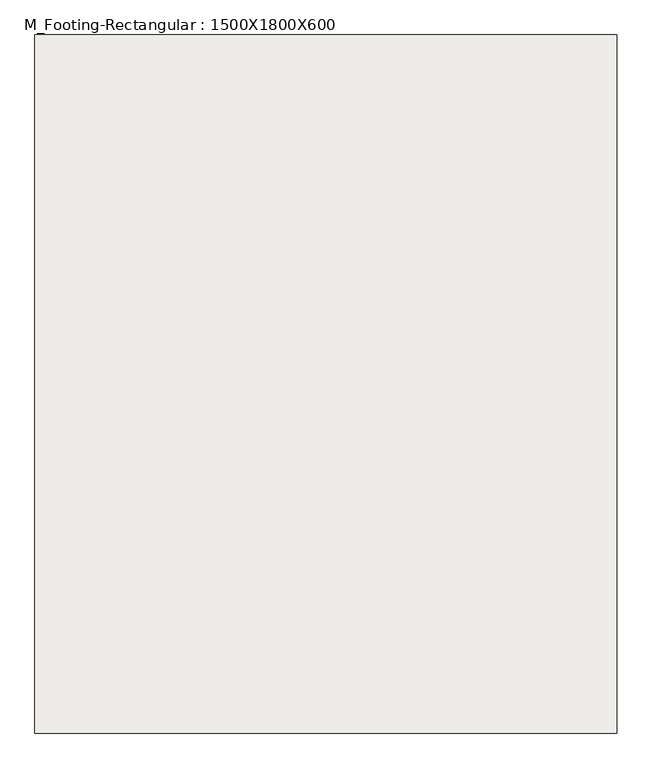
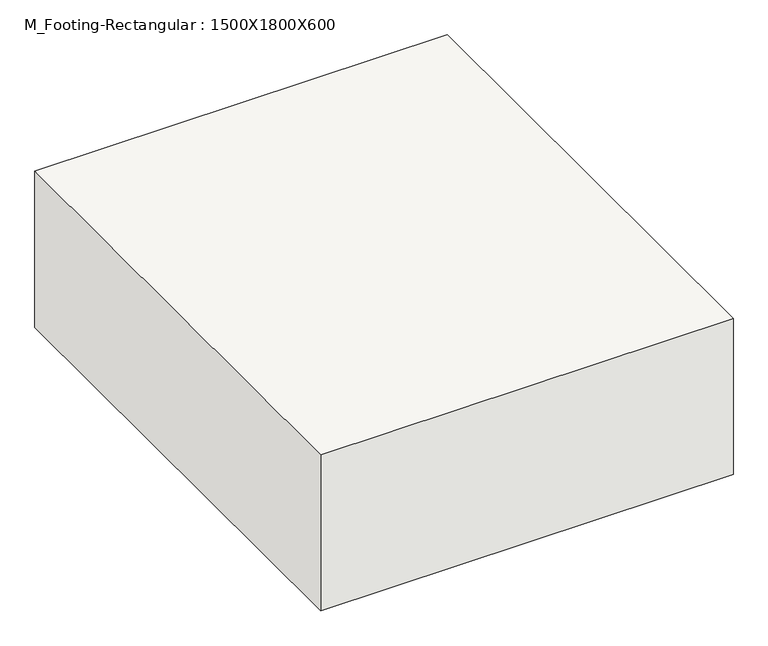
"""IFC4 building model written with IfcOpenShell, lengths in millimetres: slab geometry, M_Footing-Rectangular : 1500X1800X600."""

from ifc_helpers import new_model, si_unit, frame, origin, place, context, project, spatial, polyline, outline, extrude, source, transform, mapped, element, save


def m_footing_rectangular_1500x1800x600_40ea0b3e(model_context):
    return source(origin(), model_context, "Body", "SweptSolid", [
        extrude(outline(polyline([(750.0, 900.0), (750.0, -900.0), (-750.0, -900.0), (-750.0, 900.0), (750.0, 900.0)])), frame((0.0, 0.0, -600.0), z_axis=(0.0, 0.0, 1.0), x_axis=(1.0, 0.0, 0.0)), (0.0, 0.0, 1.0), 600.0),
    ])


if __name__ == "__main__":
    model = new_model("IFC4")
    model_context = context("Model", 3, world=origin())
    ifc_project = project(units=[si_unit("LENGTHUNIT", "METRE", prefix="MILLI")], contexts=[model_context])
    site = spatial("IfcSite", under=ifc_project)
    building = spatial("IfcBuilding", under=site)
    placement = place(None, origin())
    m_footing_rectangular_1500x1800x600_shape = m_footing_rectangular_1500x1800x600_40ea0b3e(model_context)
    element("IfcSlab", 1, ObjectType="M_Footing-Rectangular : 1500X1800X600", at=placement, inside=building, context=model_context, shape_type="MappedRepresentation", body=[
        mapped(m_footing_rectangular_1500x1800x600_shape, transform((0.0, 0.0, 0.0), x_axis=(1.0, 0.0, 0.0), y_axis=(0.0, 1.0, 0.0), z_axis=(0.0, 0.0, 1.0))),
    ])
    save(model, "model.ifc")

# Revit data of these elements
# Type "M_Footing-Rectangular : 1500X1800X600"
#   Width = 1500 mm
#   Length = 1800 mm
#   Foundation Thickness = 600 mm
#   Structural Material [instance default] = Concrete, Cast-in-Place gray
#   Assembly Code = ""
# Element 1 (IfcSlab, "M_Footing-Rectangular : 1500X1800X600")
#   Structural Material = Concrete, Cast In Situ
#   Materials on its faces: "Concrete, Cast In Situ"
# Materials
#   "Concrete, Cast-in-Place gray": class "Concrete", colour RGB 192 192 192, transparency 0, Description = "Cast-in-place concrete", Cost = 0
#   "Concrete, Cast In Situ": class "Concrete", colour RGB 192 192 192, transparency 0, Description = "physical material", Cost = 0
